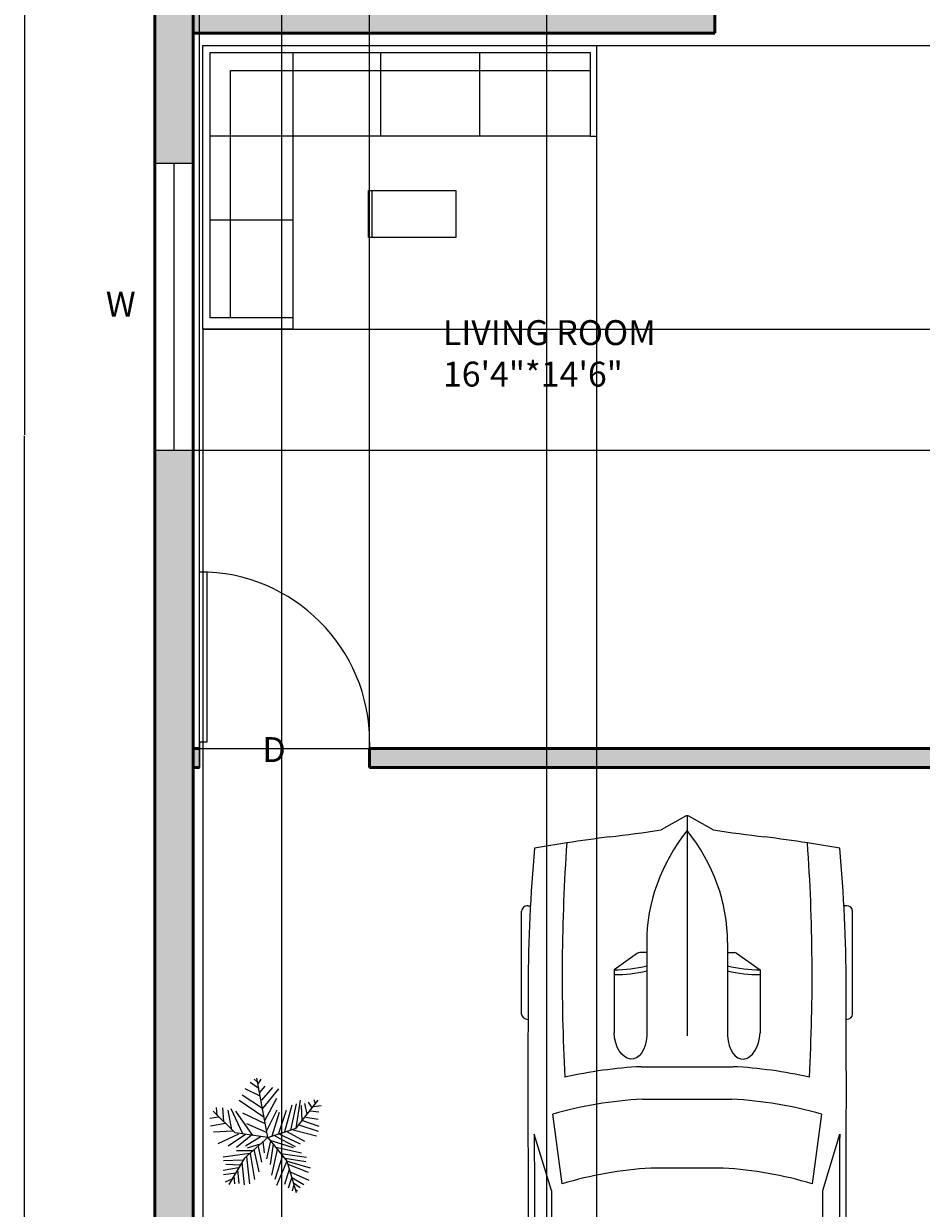
# Model space of a CAD drawing. Units: inches. Extents: x 678 to 1100, y 1432 to 2094.
# Tile 2 of 5: x 678 to 889, y 1581 to 1860. Entities that reach past the tile are written whole.
import ezdxf

# ---------------------------------------------------------------- set-up
doc = ezdxf.new("R2010")
doc.units = ezdxf.units.IN
for name, color, linetype, lineweight in [('A-ANNO-DIMS', 2, 'Continuous', 18), ('A-AREA-IDEN', 141, 'Continuous', 25), ('A-WALL-PATT', 252, 'Continuous', 13), ('C-PRKG-VEHI', 8, 'Continuous', 13), ('DOOR', 52, 'Continuous', 25), ('FUR', 30, 'Continuous', 18), ('TEXT', 141, 'Continuous', 18), ('TREE', 90, 'Continuous', 13), ('WALL', 140, 'Continuous', 50), ('WIND', 212, 'Continuous', 25)]:
    doc.layers.add(name, color=color, linetype=linetype, lineweight=lineweight)
doc.styles.get("Standard").update_dxf_attribs({"font": 'arial.ttf'})
doc.dimstyles.get("Standard").update_dxf_attribs({"dimtxt": 0.18, "dimasz": 0.18, "dimexe": 0.18, "dimexo": 0.0625, "dimgap": 0.09, "dimtad": 0, "dimtih": 1, "dimtoh": 1, "dimdec": 4, "dimzin": 0, "dimdsep": 46, "dimtxsty": 'Standard', "dimcen": 0.09, "dimadec": 0, "dimazin": 0, "dimtfac": 1, "dimtdec": 4, "dimtofl": 0, "dimtmove": 0, "dimatfit": 3, "dimfxl": 1, "dimtolj": 1, "dimtzin": 0, "dimarcsym": 0})

# ---------------------------------------------------------------- blocks, each defined once
blk = doc.blocks.new('*U8')
for p, q in [((21.1, 37.41), (21.1, 36.83)), ((46.55, 38.89), (22.35, 38.89)), ((47.8, 37.39), (47.8, 37.41)), ((135.45, 37.07), (135.45, 37.41)), ((136.7, 38.89), (160.9, 38.89)), ((162.15, 37.41), (162.15, 36.77)), ((87.99, 31.87), (74.76, 35.92)), ((134.31, 35.6), (119.29, 31.78)), ((186.47, -33.5), (186.47, 33.5)), ((70.03, 31.54), (86.41, 29.35)), ((188.4, -32.76), (188.4, 32.76)), ((138.42, 29.35), (157.25, 29.35)), ((186.47, 29.35), (167.01, 29.35)), ((164.52, 26.39), (164.52, -26.39)), ((32.27, 11.63), (36.13, 17.17)), ((36.13, 17.17), (50.94, 17.17)), ((32.12, 9.51), (32.12, 11.15)), ((29.77, 9.51), (51.68, 9.51)), ((58.92, -10.77), (58.92, 10.77)), ((66.55, -10.53), (66.55, 10.53)), ((82.74, 8.5), (82.74, -8.5)), ((186.47, -10.53), (186.47, 10.53)), ((3.27, 6.13), (0.1, 0.41)), ((0, 0), (51.68, 0)), ((0.1, -0.41), (3.27, -6.13)), ((29.77, -9.51), (51.68, -9.51)), ((32.12, -9.51), (32.12, -11.15)), ((32.27, -11.63), (36.13, -17.17)), ((36.13, -17.17), (50.94, -17.17)), ((86.41, -29.35), (70.03, -31.54)), ((157.25, -29.35), (138.42, -29.35)), ((167.01, -29.35), (186.47, -29.35)), ((87.99, -31.87), (74.76, -35.92)), ((134.31, -35.6), (119.29, -31.78)), ((21.1, -37.41), (21.1, -36.83)), ((46.55, -38.89), (22.35, -38.89)), ((47.8, -37.39), (47.8, -37.41)), ((135.45, -37.07), (135.45, -37.41)), ((136.7, -38.89), (160.9, -38.89)), ((162.15, -37.41), (162.15, -36.77))]:
    blk.add_line(p, q)
for centre, major_axis, ratio, start_param, end_param in [((41.19, -490.86), (0, 528.23), 0.842304, 0.00281, 0.075598), ((22.35, 37.41), (0, -1.48), 0.842304, 3.141593, 4.712389), ((64.48, -10555.62), (0, 10593.03), 0.842304, -0.013397, 0.002797), ((46.55, 37.41), (0, 1.48), 0.842304, -1.570796, 0), ((136.7, 37.41), (0, -1.48), 0.842304, 3.141593, 4.712389), ((160.9, 37.41), (0, 1.48), 0.842304, -1.570796, 0), ((180.63, 35.84), (0, 2.22), 0.842304, -0.013017, 1.249894), ((64.48, -10556.36), (0, 10595.31), 0.842304, -0.013397, -0.013017), ((183.98, 33.5), (0, -2.96), 0.842304, 1.570796, 3.128196), ((183.98, 32.76), (0, -5.25), 0.842304, 1.570796, 3.128196), ((266.03, -27.52), (0, 313.31), 0.842304, 1.367076, 1.39176), ((64.48, -10555.62), (0, -10591.55), 0.842304, 3.133765, 3.140441), ((135.29, 5.39), (0, 81.77), 0.842304, 1.245306, 1.50788), ((95.79, -3666.35), (0, -3698.24), 0.842304, 3.134049, 3.144098), ((259.18, -27.52), (0, -305.3), 0.842304, 4.528606, 4.561838), ((37.47, -593.96), (0, -623.33), 0.842304, 3.096046, 3.200911), ((134.4, 5.39), (0, -89.78), 0.842304, 4.449482, 4.652344), ((149.6, 2.8), (0, -79.58), 0.842304, 4.372215, 4.640744), ((17.08, 0), (0, 147.02), 0.842304, 4.511394, 4.913384), ((35.91, 0), (0, 147.02), 0.842304, 4.511394, 4.913384), ((167.01, 26.39), (0, 2.96), 0.842304, 0, 1.570796), ((-204.49, 52.4), (0, -250.96), 0.842304, 1.385369, 1.434372), ((13.04, 17.01), (0, 27.42), 0.842304, 4.435146, 4.718221), ((14.2, 17.01), (0, 27.42), 0.842304, 4.435146, 4.718221), ((50.79, 13.34), (6.34, -0.36), 0.603834, -1.395552, 1.581315), ((32.75, 11.15), (0, 0.74), 0.842304, 0.879714, 1.570796), ((29.77, -46.66), (0, 56.17), 0.842304, 0, 0.590319), ((0.62, 0), (0, -0.74), 0.842304, 4.131459, 5.293319), ((29.77, 46.66), (0, 56.17), 0.842304, 2.551274, 3.141593), ((-204.49, -52.4), (0, 250.96), 0.842304, -1.434372, -1.385369), ((13.04, -17.01), (0, -27.42), 0.842304, 1.564964, 1.848039), ((14.2, -17.01), (0, -27.42), 0.842304, 1.564964, 1.848039), ((134.4, -5.39), (0, -89.78), 0.842304, -1.510751, -1.307889), ((135.29, -5.39), (0, -81.77), 0.842304, -1.50788, -1.245306), ((149.6, -2.8), (0, -79.58), 0.842304, -1.499151, -1.230623), ((32.75, -11.15), (0, -0.74), 0.842304, 4.712389, 5.403472), ((259.18, 27.52), (0, 305.3), 0.842304, 1.721348, 1.754579), ((167.01, -26.39), (0, -2.96), 0.842304, 4.712389, 6.283185), ((266.03, 27.52), (0, 313.31), 0.842304, 1.749832, 1.774517), ((37.47, 593.96), (0, -623.33), 0.842304, -0.059319, 0.045547), ((95.79, 3666.35), (0, -3698.24), 0.842304, -0.002505, 0.007544), ((183.98, -32.76), (0, -5.25), 0.842304, 0.013397, 1.570796), ((41.19, 490.86), (0, -528.23), 0.842304, -0.075598, -0.00281), ((64.48, 10555.62), (0, -10591.55), 0.842304, 0.001152, 0.007828), ((183.98, -33.5), (0, 2.96), 0.842304, 3.15499, 4.712389), ((22.35, -37.41), (0, 1.48), 0.842304, 1.570796, 3.141593), ((64.48, 10555.62), (0, 10593.03), 0.842304, 3.138796, 3.15499), ((46.55, -37.41), (0, -1.48), 0.842304, 0, 1.570796), ((136.7, -37.41), (0, -1.48), 0.842304, -1.570796, 0), ((160.9, -37.41), (0, 1.48), 0.842304, 3.141593, 4.712389), ((180.63, -35.84), (0, -2.22), 0.842304, -1.249894, 0.013017), ((64.48, 10556.36), (0, 10595.31), 0.842304, 3.15461, 3.15499)]:
    blk.add_ellipse(centre, major_axis=major_axis, ratio=ratio, start_param=start_param, end_param=end_param)
at = {"extrusion": (0, 0, -1)}
blk.add_ellipse((50.79, -13.34), major_axis=(6.34, 0.36), ratio=0.603834, start_param=-1.395552, end_param=1.581315, dxfattribs=at)
blk = doc.blocks.new('*U2')
for p, q in [((0, 0), (0, -6)), ((40, 0), (40, -6))]:
    blk.add_line(p, q)
blk.add_lwpolyline([(0, 0), (0, 40), (1.75, 40), (1.75, 0)], close=True)
blk.add_arc((0, 0), 40, 0, 90)
blk = doc.blocks.new('*U6')
for p, q in [((0, 0), (-10.5, 57)), ((-7.288, 39.707), (-21.778, 46.673)), ((-8.737, 47.138), (-17.069, 52.711)), ((-10.186, 53.64), (-13.084, 55.962)), ((-9.099, 51.782), (-6.563, 55.962)), ((-7.65, 43.423), (-2.578, 49.46)), ((-5.839, 35.992), (4.667, 48.067)), ((-5.114, 27.632), (10.463, 46.673)), ((-3.665, 19.273), (-27.574, 35.527)), ((-5.114, 28.097), (-24.676, 40.636)), ((-2.941, 16.486), (8.652, 37.85)), ((27, 9), (48, 36)), ((27.127, 9.056), (31.112, 35.992)), ((38.719, 34.134), (41.979, 28.561)), ((44.153, 36.456), (45.239, 32.741)), ((-31.5, 4.5), (-52.5, 25.5)), ((-48.585, 21.131), (-49.309, 29.026)), ((-43.513, 28.561), (-42.427, 15.558)), ((-38.442, 26.239), (-34.819, 7.663)), ((-35.544, 28.097), (-24.314, 3.947)), ((-14.533, 2.09), (-30.834, 25.31)), ((-24.314, 23.917), (-2.941, 13.7)), ((-1.129, 6.734), (9.014, 26.704)), ((3.942, 1.625), (11.187, 24.381)), ((10.101, 3.483), (17.708, 26.239)), ((16.259, 5.805), (23.142, 31.348)), ((22.055, 7.198), (27.489, 32.277)), ((31.836, 30.883), (32.561, 16.486)), ((35.096, 32.741), (37.27, 22.524)), ((40.53, 25.775), (48.862, 24.846)), ((43.791, 29.954), (51.036, 30.883)), ((-47.498, 19.737), (-55.83, 18.344)), ((-40.615, 13.7), (-55.105, 10.913)), ((-20.691, 13.7), (-1.129, 4.876)), ((29.662, 12.307), (48.137, 6.269)), ((33.285, 16.486), (48.862, 10.913)), ((36.183, 19.737), (48.137, 17.88)), ((-33.37, 6.269), (-52.207, 5.34)), ((-28.299, 3.483), (-47.86, -5.805)), ((-21.416, 3.018), (-38.079, -8.128)), ((0, 0), (-31.5, 4.5)), ((-15.982, 2.09), (-30.11, -9.521)), ((0, 0), (-22.5, -19.5)), ((-6.563, 1.161), (-21.416, -8.128)), ((0, 0), (27, 9)), ((0, 0), (18, -22.5)), ((6.478, 1.625), (26.04, -8.592)), ((11.187, 3.483), (30.749, -5.805)), ((18.07, 5.805), (35.096, -3.483)), ((24.229, 7.663), (46.688, 1.625)), ((-6.563, -5.805), (-19.967, -9.985)), ((-9.461, -8.592), (-6.201, -23.453)), ((-4.752, -3.483), (-3.665, -14.629)), ((2.493, -3.019), (-1.491, -20.202)), ((1.769, -2.555), (24.229, -9.521)), ((5.029, -6.27), (2.131, -25.775)), ((7.565, -9.056), (32.198, -14.629)), ((-17.431, -15.094), (-42.789, -18.809)), ((-24.314, -21.596), (-42.427, -22.06)), ((-22.5, -19.5), (-37.5, -45)), ((-15.257, -12.772), (-30.11, -12.772)), ((-20.691, -18.345), (-17.793, -44.352)), ((-17.069, -15.094), (-12.721, -40.172)), ((-13.446, -11.378), (-8.737, -32.741)), ((9.014, -11.378), (3.58, -35.992)), ((14.085, -16.951), (6.478, -40.172)), ((18.07, -22.524), (8.289, -45.745)), ((12.274, -15.094), (36.907, -18.809)), ((16.259, -19.738), (36.183, -22.989)), ((18, -22.5), (27, -52.5)), ((18.433, -22.524), (40.53, -29.026)), ((-28.299, -29.026), (-42.789, -31.348)), ((-26.849, -26.24), (-40.253, -25.775)), ((-29.023, -30.884), (-27.936, -43.887)), ((-25.038, -23.918), (-22.865, -45.281)), ((20.244, -30.419), (15.897, -44.816)), ((19.157, -25.311), (38.719, -33.206)), ((21.331, -32.741), (39.081, -40.636)), ((-30.834, -34.135), (-42.427, -35.528)), ((-34.457, -39.708), (-40.978, -42.494)), ((-32.646, -36.921), (-31.921, -44.352)), ((22.78, -37.85), (19.519, -48.532)), ((22.78, -38.314), (34.372, -44.816)), ((24.591, -43.423), (30.749, -47.603)), ((24.591, -45.745), (23.142, -50.854)), ((26.764, -49.925), (28.213, -50.854))]:
    blk.add_line(p, q)
blk = doc.blocks.new('WIN-STANDARD')
blk.add_line((4.5, 0), (4.5, 67.31))
blk.add_lwpolyline([(9, 67.31), (0, 67.31), (0, 0), (9, 0)], close=True)
blk = doc.blocks.new('*D25')
at = {"layer": 'A-ANNO-DIMS', "color": 0, "lineweight": -2, "transparency": 16777216}
for p, q in [((708.9, 2062.93), (678.13, 2062.93)), ((678.31, 2062.75), (678.31, 1763.11)), ((678.31, 1463.11), (678.31, 1762.75)), ((708.9, 1462.93), (678.13, 1462.93))]:
    blk.add_line(p, q, dxfattribs=at)
at = {"layer": 'A-ANNO-DIMS', "color": 0, "transparency": 16777216}
for points in [[(678.28, 2062.75), (678.34, 2062.75), (678.31, 2062.93)], [(678.28, 1463.11), (678.34, 1463.11), (678.31, 1462.93)]]:
    blk.add_solid(points, dxfattribs=at)
at = {"layer": 'Defpoints', "color": 0, "transparency": 16777216}
for p in [(678.31, 2062.93), (708.96, 2062.93), (708.96, 1462.93)]:
    blk.add_point(p, dxfattribs=at)
at = {"layer": 'A-ANNO-DIMS', "color": 0, "transparency": 16777216, "insert": (678.31, 1762.93), "char_height": 0.18, "attachment_point": 5}
blk.add_mtext('\\A1;600', dxfattribs=at)
blk = doc.blocks.new('*D41')
at = {"layer": 'A-ANNO-DIMS', "color": 0, "lineweight": -2, "transparency": 16777216}
for p, q in [((718.02, 1759.52), (1099.79, 1759.52)), ((1099.61, 1759.34), (1099.61, 1724.66)), ((1099.61, 1689.61), (1099.61, 1724.29)), ((718.02, 1689.43), (1099.79, 1689.43))]:
    blk.add_line(p, q, dxfattribs=at)
at = {"layer": 'A-ANNO-DIMS', "color": 0, "transparency": 16777216}
for points in [[(1099.58, 1759.34), (1099.64, 1759.34), (1099.61, 1759.52)], [(1099.58, 1689.61), (1099.64, 1689.61), (1099.61, 1689.43)]]:
    blk.add_solid(points, dxfattribs=at)
at = {"layer": 'Defpoints', "color": 0, "transparency": 16777216}
for p in [(717.96, 1759.52), (1099.61, 1759.52), (717.96, 1689.43)]:
    blk.add_point(p, dxfattribs=at)
at = {"layer": 'A-ANNO-DIMS', "color": 0, "transparency": 16777216, "insert": (1099.61, 1724.48), "char_height": 0.18, "attachment_point": 5}
blk.add_mtext('\\A1;70.1', dxfattribs=at)
blk = doc.blocks.new('*D45')
at = {"layer": 'A-ANNO-DIMS', "color": 0, "lineweight": -2, "transparency": 16777216}
for p, q in [((719.41, 1684.99), (719.41, 2093.76)), ((719.59, 2093.58), (739.19, 2093.58)), ((759.23, 2093.58), (739.63, 2093.58)), ((759.41, 1684.99), (759.41, 2093.76))]:
    blk.add_line(p, q, dxfattribs=at)
at = {"layer": 'A-ANNO-DIMS', "color": 0, "transparency": 16777216}
for points in [[(719.59, 2093.61), (719.59, 2093.55), (719.41, 2093.58)], [(759.23, 2093.61), (759.23, 2093.55), (759.41, 2093.58)]]:
    blk.add_solid(points, dxfattribs=at)
at = {"layer": 'Defpoints', "color": 0, "transparency": 16777216}
for p in [(759.41, 2093.58), (719.41, 1684.93), (759.41, 1684.93)]:
    blk.add_point(p, dxfattribs=at)
at = {"layer": 'A-ANNO-DIMS', "color": 0, "transparency": 16777216, "insert": (739.41, 2093.58), "char_height": 0.18, "attachment_point": 5}
blk.add_mtext('\\A1;40', dxfattribs=at)
blk = doc.blocks.new('*D53')
at = {"layer": 'A-ANNO-DIMS', "color": 0, "lineweight": -2, "transparency": 16777216}
for p, q in [((738.71, 1897.06), (738.71, 1432.1)), ((800.95, 1897.06), (800.95, 1432.1)), ((738.89, 1432.28), (769.43, 1432.28)), ((800.77, 1432.28), (770.22, 1432.28))]:
    blk.add_line(p, q, dxfattribs=at)
at = {"layer": 'A-ANNO-DIMS', "color": 0, "transparency": 16777216}
for points in [[(738.89, 1432.31), (738.89, 1432.25), (738.71, 1432.28)], [(800.77, 1432.31), (800.77, 1432.25), (800.95, 1432.28)]]:
    blk.add_solid(points, dxfattribs=at)
at = {"layer": 'Defpoints', "color": 0, "transparency": 16777216}
for p in [(738.71, 1897.12), (800.95, 1897.12), (800.95, 1432.28)]:
    blk.add_point(p, dxfattribs=at)
at = {"layer": 'A-ANNO-DIMS', "color": 0, "transparency": 16777216, "insert": (769.83, 1432.28), "char_height": 0.18, "attachment_point": 5}
blk.add_mtext('\\A1;62.25', dxfattribs=at)
blk = doc.blocks.new('*D55')
at = {"layer": 'A-ANNO-DIMS', "color": 0, "lineweight": -2, "transparency": 16777216}
for p, q in [((812.72, 1833.21), (812.72, 1432.1)), ((720.22, 1787.87), (720.22, 1432.1)), ((720.4, 1432.28), (766.15, 1432.28)), ((812.54, 1432.28), (766.8, 1432.28))]:
    blk.add_line(p, q, dxfattribs=at)
at = {"layer": 'A-ANNO-DIMS', "color": 0, "transparency": 16777216}
for points in [[(720.4, 1432.31), (720.4, 1432.25), (720.22, 1432.28)], [(812.54, 1432.31), (812.54, 1432.25), (812.72, 1432.28)]]:
    blk.add_solid(points, dxfattribs=at)
at = {"layer": 'Defpoints', "color": 0, "transparency": 16777216}
for p in [(812.72, 1833.27), (720.22, 1787.94), (812.72, 1432.28)]:
    blk.add_point(p, dxfattribs=at)
at = {"layer": 'A-ANNO-DIMS', "color": 0, "transparency": 16777216, "insert": (766.47, 1432.28), "char_height": 0.18, "attachment_point": 5}
blk.add_mtext('\\A1;92.5', dxfattribs=at)
blk = doc.blocks.new('*D56')
at = {"layer": 'A-ANNO-DIMS', "color": 0, "lineweight": -2, "transparency": 16777216}
for p, q in [((720.28, 1854.56), (1099.79, 1854.56)), ((1099.61, 1854.38), (1099.61, 1821.43)), ((1099.61, 1788.12), (1099.61, 1821.06)), ((720.28, 1787.94), (1099.79, 1787.94))]:
    blk.add_line(p, q, dxfattribs=at)
at = {"layer": 'A-ANNO-DIMS', "color": 0, "transparency": 16777216}
for points in [[(1099.58, 1854.38), (1099.64, 1854.38), (1099.61, 1854.56)], [(1099.58, 1788.12), (1099.64, 1788.12), (1099.61, 1787.94)]]:
    blk.add_solid(points, dxfattribs=at)
at = {"layer": 'Defpoints', "color": 0, "transparency": 16777216}
for p in [(720.22, 1854.56), (1099.61, 1854.56), (720.22, 1787.94)]:
    blk.add_point(p, dxfattribs=at)
at = {"layer": 'A-ANNO-DIMS', "color": 0, "transparency": 16777216, "insert": (1099.61, 1821.25), "char_height": 0.18, "attachment_point": 5}
blk.add_mtext('\\A1;66.62', dxfattribs=at)

msp = doc.modelspace()

# ---------------------------------------------------------------- hatches: boundary and pattern name
at = {"layer": 'A-WALL-PATT'}
h = msp.add_hatch(color=256, dxfattribs=at)
h.dxf.hatch_style = 1
h.paths.add_polyline_path([(859.7133, 2062.9286), (708.9606, 2062.9286), (708.9606, 2031.3203), (717.9606, 2031.3203), (717.9606, 2053.9286), (837.9606, 2053.9286), (859.7133, 2053.9286)])
h.paths.add_polyline_path([(957.0069, 2062.9286), (896.0724, 2062.9286), (896.0724, 2053.9286), (957.0069, 2053.9286)])
h.paths.add_polyline_path([(842.4606, 2053.9286), (837.9606, 2053.9286), (837.9606, 2005.4286), (842.4606, 2005.4286), (923.4606, 2005.4286), (923.4606, 2009.9286), (842.4606, 2009.9286)])
h.paths.add_polyline_path([(927.9606, 2053.9286), (923.4606, 2053.9286), (923.4606, 2052.1286), (924.8103, 2052.1286), (927.9606, 2052.1286)])
h.paths.add_polyline_path([(1068.9606, 2062.9286), (1024.3184, 2062.9286), (1024.3184, 2053.9286), (1028.6041, 2053.9286), (1059.9606, 2053.9286), (1059.9606, 2002.6361), (1068.9606, 2002.6361)])
h.paths.add_polyline_path([(1059.9606, 1861.9286), (996.9604, 1861.9286), (927.9606, 1861.9286), (923.4606, 1861.9286), (923.4606, 1857.4286), (1059.9606, 1857.4286)], flags=17)
h.paths.add_polyline_path([(927.9606, 2031.1269), (924.8103, 2031.1269, -0.01607952), (923.4606, 2031.1703), (923.4606, 1905.3856), (927.9606, 1905.3856)])
h.paths.add_polyline_path([(923.4606, 1957.9286), (842.4606, 1957.9286), (842.4606, 1969.339), (837.9606, 1969.339), (837.9606, 1953.4286), (923.4606, 1953.4286)])
h.paths.add_polyline_path([(774.6357, 1957.9286), (717.9606, 1957.9286), (717.9606, 1953.4286), (774.6357, 1953.4286)])
h.paths.add_polyline_path([(717.9606, 1979.9404), (708.9606, 1979.9404), (708.9606, 1945.1463), (717.9606, 1945.1463)])
h.paths.add_polyline_path([(840.5596, 1861.9286), (717.9606, 1861.9286), (717.9606, 1857.4286), (840.5596, 1857.4286)], flags=17)
h.paths.add_polyline_path([(927.9606, 1865.3856), (923.4606, 1865.3856), (923.4606, 1861.9286), (927.9606, 1861.9286)], flags=17)
h.paths.add_polyline_path([(1059.9606, 1689.4286), (967.3461, 1689.4286), (967.3461, 1684.9286), (1059.9606, 1684.9286)], flags=17)
h.paths.add_polyline_path([(987.9606, 1737.4286), (983.4606, 1737.4286), (983.4606, 1715.196), (986.7357, 1715.196, -0.01403382), (987.9606, 1715.1616)], flags=17)
h.paths.add_polyline_path([(916.0499, 2036.8414), (924.8721, 2036.8414), (924.8721, 2048.8901), (916.0499, 2048.8901)], flags=9)
h.paths.add_polyline_path([(921.7778, 1883.2914), (930.5999, 1883.2914), (930.5999, 1895.3401), (921.7778, 1895.3401)], flags=25)
h.paths.add_polyline_path([(732.1085, 1683.0506), (740.9307, 1683.0506), (740.9307, 1695.0993), (732.1085, 1695.0993)], flags=25)
h.paths.add_polyline_path([(943.8458, 1737.5114), (952.6679, 1737.5114), (952.6679, 1749.5601), (943.8458, 1749.5601)], flags=25)
h.paths.add_polyline_path([(986.0751, 1696.9795), (994.8973, 1696.9795), (994.8973, 1709.0282), (986.0751, 1709.0282)], flags=25)
h.paths.add_polyline_path([(940.1881, 1677.378), (949.0103, 1677.378), (949.0103, 1689.4267), (940.1881, 1689.4267)], flags=25)
h.paths.add_polyline_path([(998.6262, 1761.7469), (1044.0453, 1761.7469), (1044.0453, 1783.5644), (998.6262, 1783.5644)], flags=25)
h.paths.add_polyline_path([(997.3001, 1713.4735), (1028.9316, 1713.4735), (1028.9316, 1735.2909), (997.3001, 1735.2909)], flags=25)
h.paths.add_polyline_path([(1005.9896, 1586.8139), (1051.4087, 1586.8139), (1051.4087, 1608.6313), (1005.9896, 1608.6313)], flags=25)
h.paths.add_polyline_path([(794.7038, 1552.8124), (873.8721, 1552.8124), (873.8721, 1574.6298), (794.7038, 1574.6298)], flags=25)
h.paths.add_polyline_path([(774.2693, 1771.1228), (831.9444, 1771.1228), (831.9444, 1792.9403), (774.2693, 1792.9403)], flags=25)
h.paths.add_polyline_path([(750.0357, 1897.1514), (786.4291, 1897.1514), (786.4291, 1918.9689), (750.0357, 1918.9689)], flags=25)
h.paths.add_polyline_path([(974.9086, 1953.7921), (1020.3276, 1953.7921), (1020.3276, 1975.6096), (974.9086, 1975.6096)], flags=9)
h.paths.add_polyline_path([(859.1564, 1973.8092), (890.2175, 1973.8092), (890.2175, 1995.6267), (859.1564, 1995.6267)], flags=9)
h.paths.add_polyline_path([(753.2305, 1989.0219), (792.2962, 1989.0219), (792.2962, 2010.8393), (753.2305, 2010.8393)], flags=9)
h.paths.add_polyline_path([(1067.3992, 1620.1515), (1078.032, 1620.1515), (1078.032, 1632.2002), (1067.3992, 1632.2002)], flags=9)
h.paths.add_polyline_path([(846.8446, 2028.8178), (878.5079, 2028.8178), (878.5079, 2050.6353), (846.8446, 2050.6353)], flags=25)
h.paths.add_polyline_path([(1059.9606, 1832.7202), (1068.9606, 1832.7202), (1068.9606, 1935.3246), (1059.9606, 1935.3246)])
h.paths.add_polyline_path([(1068.9606, 1765.4088), (1059.9606, 1765.4088), (1059.9606, 1728.1446), (1068.9606, 1728.1446)])
h.paths.add_polyline_path([(1059.9606, 1657.7018), (1068.9606, 1657.7018), (1068.9606, 1697.8017), (1059.9606, 1697.8017)])
h.paths.add_polyline_path([(1068.9606, 1590.3903), (1059.9606, 1590.3903), (1059.9606, 1551.1623), (1068.9606, 1551.1623)])
h.paths.add_polyline_path([(708.9606, 1826.8331), (717.9606, 1826.8331), (717.9606, 1877.8348), (708.9606, 1877.8348)])
h.paths.add_polyline_path([(717.9606, 1759.5217), (708.9606, 1759.5217), (708.9606, 1462.9286), (1068.9606, 1462.9286), (1068.9606, 1483.8508), (1059.9606, 1483.8508), (1059.9606, 1471.9286), (717.9606, 1471.9286)])
h = msp.add_hatch(color=256, dxfattribs=at)
h.dxf.hatch_style = 1
h.paths.add_polyline_path([(1059.9606, 1741.9286), (970.7942, 1741.9286), (970.7942, 1737.4286), (1059.9606, 1737.4286)])
h.paths.add_polyline_path([(927.3461, 1689.4286), (759.4099, 1689.4286), (759.4099, 1684.9286), (927.3461, 1684.9286)])
h.paths.add_polyline_path([(921.9606, 1684.9286), (917.4606, 1684.9286), (917.4606, 1560.4286), (921.9606, 1560.4286)])
h.paths.add_polyline_path([(1059.9606, 1564.9286), (921.9606, 1564.9286), (921.9606, 1560.4286), (1059.9606, 1560.4286)])
h.paths.add_polyline_path([(916.0499, 2036.8414), (924.8721, 2036.8414), (924.8721, 2048.8901), (916.0499, 2048.8901)], flags=9)
h.paths.add_polyline_path([(921.7778, 1883.2914), (930.5999, 1883.2914), (930.5999, 1895.3401), (921.7778, 1895.3401)], flags=9)
h.paths.add_polyline_path([(732.1085, 1683.0506), (740.9307, 1683.0506), (740.9307, 1695.0993), (732.1085, 1695.0993)], flags=9)
h.paths.add_polyline_path([(943.8458, 1737.5114), (952.6679, 1737.5114), (952.6679, 1749.5601), (943.8458, 1749.5601)], flags=9)
h.paths.add_polyline_path([(986.0751, 1696.9795), (994.8973, 1696.9795), (994.8973, 1709.0282), (986.0751, 1709.0282)], flags=9)
h.paths.add_polyline_path([(940.1881, 1677.378), (949.0103, 1677.378), (949.0103, 1689.4267), (940.1881, 1689.4267)], flags=9)
h.paths.add_polyline_path([(998.6262, 1761.7469), (1044.0453, 1761.7469), (1044.0453, 1783.5644), (998.6262, 1783.5644)], flags=9)
h.paths.add_polyline_path([(1005.9896, 1586.8139), (1051.4087, 1586.8139), (1051.4087, 1608.6313), (1005.9896, 1608.6313)], flags=9)
h.paths.add_polyline_path([(794.7038, 1552.8124), (873.8721, 1552.8124), (873.8721, 1574.6298), (794.7038, 1574.6298)], flags=9)
h.paths.add_polyline_path([(774.2693, 1771.1228), (831.9444, 1771.1228), (831.9444, 1792.9403), (774.2693, 1792.9403)], flags=9)
h.paths.add_polyline_path([(750.0357, 1897.1514), (786.4291, 1897.1514), (786.4291, 1918.9689), (750.0357, 1918.9689)], flags=9)
h.paths.add_polyline_path([(974.9086, 1953.7921), (1020.3276, 1953.7921), (1020.3276, 1975.6096), (974.9086, 1975.6096)], flags=9)
h.paths.add_polyline_path([(859.1564, 1973.8092), (890.2175, 1973.8092), (890.2175, 1995.6267), (859.1564, 1995.6267)], flags=9)
h.paths.add_polyline_path([(846.8446, 2028.8178), (878.5079, 2028.8178), (878.5079, 2050.6353), (846.8446, 2050.6353)], flags=9)
h.paths.add_polyline_path([(753.2305, 1989.0219), (792.2962, 1989.0219), (792.2962, 2010.8393), (753.2305, 2010.8393)], flags=9)
h = msp.add_hatch(color=256, dxfattribs=at)
h.dxf.hatch_style = 1
h.paths.add_polyline_path([(927.9606, 1857.4286), (923.4606, 1857.4286), (923.4606, 1737.4286), (927.9606, 1737.4286)])
h.paths.add_polyline_path([(930.7942, 1741.9286), (927.9606, 1741.9286), (927.9606, 1737.4286), (930.7942, 1737.4286)])
h.paths.add_polyline_path([(916.0499, 2036.8414), (924.8721, 2036.8414), (924.8721, 2048.8901), (916.0499, 2048.8901)], flags=9)
h.paths.add_polyline_path([(921.7778, 1883.2914), (930.5999, 1883.2914), (930.5999, 1895.3401), (921.7778, 1895.3401)], flags=9)
h.paths.add_polyline_path([(732.1085, 1683.0506), (740.9307, 1683.0506), (740.9307, 1695.0993), (732.1085, 1695.0993)], flags=9)
h.paths.add_polyline_path([(943.8458, 1737.5114), (952.6679, 1737.5114), (952.6679, 1749.5601), (943.8458, 1749.5601)], flags=9)
h.paths.add_polyline_path([(986.0751, 1696.9795), (994.8973, 1696.9795), (994.8973, 1709.0282), (986.0751, 1709.0282)], flags=9)
h.paths.add_polyline_path([(940.1881, 1677.378), (949.0103, 1677.378), (949.0103, 1689.4267), (940.1881, 1689.4267)], flags=9)
h.paths.add_polyline_path([(998.6262, 1761.7469), (1044.0453, 1761.7469), (1044.0453, 1783.5644), (998.6262, 1783.5644)], flags=9)
h.paths.add_polyline_path([(997.3001, 1713.4735), (1028.9316, 1713.4735), (1028.9316, 1735.2909), (997.3001, 1735.2909)], flags=9)
h.paths.add_polyline_path([(1005.9896, 1586.8139), (1051.4087, 1586.8139), (1051.4087, 1608.6313), (1005.9896, 1608.6313)], flags=9)
h.paths.add_polyline_path([(794.7038, 1552.8124), (873.8721, 1552.8124), (873.8721, 1574.6298), (794.7038, 1574.6298)], flags=9)
h.paths.add_polyline_path([(774.2693, 1771.1228), (831.9444, 1771.1228), (831.9444, 1792.9403), (774.2693, 1792.9403)], flags=9)
h.paths.add_polyline_path([(750.0357, 1897.1514), (786.4291, 1897.1514), (786.4291, 1918.9689), (750.0357, 1918.9689)], flags=9)
h.paths.add_polyline_path([(974.9086, 1953.7921), (1020.3276, 1953.7921), (1020.3276, 1975.6096), (974.9086, 1975.6096)], flags=9)
h.paths.add_polyline_path([(859.1564, 1973.8092), (890.2175, 1973.8092), (890.2175, 1995.6267), (859.1564, 1995.6267)], flags=9)
h.paths.add_polyline_path([(846.8446, 2028.8178), (878.5079, 2028.8178), (878.5079, 2050.6353), (846.8446, 2050.6353)], flags=9)
h.paths.add_polyline_path([(753.2305, 1989.0219), (792.2962, 1989.0219), (792.2962, 2010.8393), (753.2305, 2010.8393)], flags=9)
h = msp.add_hatch(color=256, dxfattribs=at)
h.dxf.hatch_style = 1
h.paths.add_polyline_path([(719.4099, 1689.4286), (717.9606, 1689.4286), (717.9606, 1684.9286), (719.4099, 1684.9286)])

# ---------------------------------------------------------------- linework, layer by layer
at = {"layer": 'FUR'}
for p, q in [((720.2201, 1787.9351), (720.2201, 1854.5558)), ((720.2201, 1854.5558), (812.7228, 1854.5558)), ((812.7228, 1854.5558), (812.7228, 1833.2731)), ((761.9278, 1852.9006), (761.9278, 1833.2731)), ((785.1833, 1852.9006), (785.1833, 1833.2731)), ((726.7159, 1790.5739), (726.7159, 1848.6629)), ((726.7159, 1848.6629), (811.2367, 1848.6629)), ((811.2367, 1833.2731), (812.7228, 1833.2731)), ((759.8965, 1820.5036), (759.8965, 1809.4408)), ((721.9289, 1813.6434), (741.3301, 1813.6434)), ((741.3301, 1790.5739), (741.3301, 1787.9351)), ((741.3301, 1787.9351), (720.2201, 1787.9351))]:
    msp.add_line(p, q, dxfattribs=at)
for points in [[(721.9289, 1852.9006), (811.2367, 1852.9006), (811.2367, 1833.2731), (721.9289, 1833.2731)], [(721.9289, 1852.9006), (741.3301, 1852.9006), (741.3301, 1790.5739), (721.9289, 1790.5739)], [(759.1701, 1820.5036), (779.6373, 1820.5036), (779.6373, 1809.4408), (759.1701, 1809.4408)]]:
    msp.add_lwpolyline(points, close=True, dxfattribs=at)
at = {"layer": 'WALL'}
for p, q in [((708.9606, 1462.9286), (708.9606, 2062.9286)), ((840.5596, 1861.9286), (840.5596, 1857.4286)), ((840.5596, 1857.4286), (717.9606, 1857.4286)), ((717.9606, 1471.9286), (717.9606, 1708.9286)), ((719.4099, 1689.4286), (717.9606, 1689.4286)), ((917.4606, 1689.4286), (759.4099, 1689.4286)), ((719.4099, 1684.9286), (717.9606, 1684.9286)), ((921.9606, 1684.9286), (759.4099, 1684.9286))]:
    msp.add_line(p, q, dxfattribs=at)
for points in [[(708.9606, 2062.9286), (1068.9606, 2062.9286), (1068.9606, 1462.9286), (708.9606, 1462.9286)], [(717.9606, 2053.9286), (1059.9606, 2053.9286), (1059.9606, 1471.9286), (717.9606, 1471.9286)], [(759.4099, 1684.9286), (927.3461, 1684.9286), (927.3461, 1689.4286), (759.4099, 1689.4286)]]:
    msp.add_lwpolyline(points, close=True, dxfattribs=at)

# ---------------------------------------------------------------- block references
at = {"layer": 'C-PRKG-VEHI', "rotation": 270}
msp.add_blockref('*U8', (834.016, 1673.5922), dxfattribs=at)
at = {"layer": 'DOOR'}
msp.add_blockref('*U2', (719.4099, 1690.9286), dxfattribs=at)
at = {"layer": 'TREE', "xscale": 0.2451816363405065, "yscale": 0.2451816363405065, "zscale": 0.2451816363405065}
msp.add_blockref('*U6', (735.5015, 1598.0074), dxfattribs=at)
at = {"layer": 'WIND'}
msp.add_blockref('WIN-STANDARD', (708.961, 1759.5218), dxfattribs=at)

# ---------------------------------------------------------------- texts
at = {"layer": 'A-AREA-IDEN', "insert": (776.6204, 1790.0348), "char_height": 5.846885, "attachment_point": 1}
msp.add_mtext_dynamic_manual_height_columns('LIVING ROOM\\P16\'4"*14\'6"', width=180.890738, gutter_width=29.2344, heights=[0], dxfattribs=at)
at = {"layer": 'TEXT', "char_height": 5.8469, "attachment_point": 1}
for s, insert in [('W', (697.4089, 1796.744)), ('D', (734.2004, 1692.0902))]:
    msp.add_mtext_dynamic_manual_height_columns(s, width=180.890738, gutter_width=29.2344, heights=[0], dxfattribs=dict(at, insert=insert))

# ---------------------------------------------------------------- dimensions: what is measured, and where the dimension line sits
at = {"layer": 'A-ANNO-DIMS'}
for base, p1, p2, override, picture, middle in [((759.4099, 2093.5786), (719.4099, 1684.9286), (759.4099, 1684.9286), {"dimdec": 0, "dimlfac": 1, "dimrnd": 0, "dimzin": 0, "dimdsep": 46, "dimlunit": 2}, '*D45', (739.4099, 2093.5786)), ((800.9505, 1432.2786), (738.7053, 1897.12), (800.9505, 1897.12), {"dimdec": 2, "dimlfac": 1, "dimrnd": 0, "dimzin": 0, "dimdsep": 46, "dimlunit": 2}, '*D53', (769.8279, 1432.2786)), ((812.7228, 1432.2786), (720.2201, 1787.9351), (812.7228, 1833.2731), {"dimdec": 1, "dimlfac": 1, "dimrnd": 0, "dimzin": 0, "dimdsep": 46, "dimlunit": 2}, '*D55', (766.4715, 1432.2786))]:
    dim = msp.add_linear_dim(base=base, p1=p1, p2=p2, dimstyle='Standard', override=override, dxfattribs=at)
    dim.commit()
    dim.dimension.update_dxf_attribs({"geometry": picture, "text_midpoint": middle})
for base, p1, p2, override, picture, middle in [((678.3106, 2062.9286), (708.9606, 1462.9286), (708.9606, 2062.9286), {"dimdec": 0, "dimlfac": 1, "dimrnd": 0, "dimzin": 0, "dimdsep": 46, "dimlunit": 2}, '*D25', (678.3106, 1762.9286)), ((1099.6106, 1854.5558), (720.2201, 1787.9351), (720.2201, 1854.5558), {"dimdec": 2, "dimlfac": 1, "dimrnd": 0, "dimzin": 0, "dimdsep": 46, "dimlunit": 2}, '*D56', (1099.6106, 1821.2455)), ((1099.6106, 1759.5217), (717.9606, 1689.4286), (717.9606, 1759.5217), {"dimdec": 1, "dimlfac": 1, "dimrnd": 0, "dimzin": 0, "dimdsep": 46, "dimlunit": 2}, '*D41', (1099.6106, 1724.4751))]:
    dim = msp.add_linear_dim(base=base, p1=p1, p2=p2, angle=90, dimstyle='Standard', override=override, dxfattribs=at)
    dim.commit()
    dim.dimension.update_dxf_attribs({"geometry": picture, "text_midpoint": middle})

doc.saveas('drawing.dxf')
